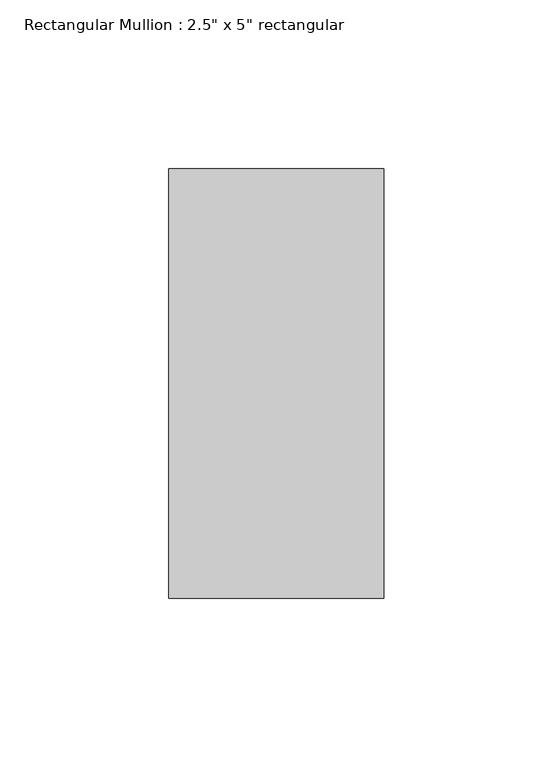
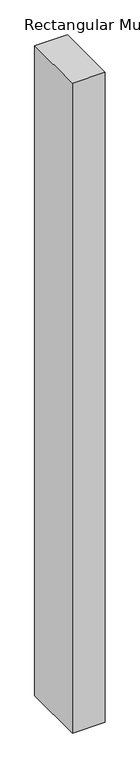
"""IFC4 building model written with IfcOpenShell, lengths in millimetres: member geometry."""

from ifc_helpers import new_model, si_unit, frame, origin, place, context, project, spatial, polyline, outline, extrude, source, transform, mapped, element, save


def member_abf390f1(model_context):
    return source(origin(), model_context, "Body", "SweptSolid", [
        extrude(outline(polyline([(0.0, 63.5), (0.0, -63.5), (-63.5, -63.5), (-63.5, 63.5), (0.0, 63.5)])), frame((0.0, 0.0, -1333.4999998), z_axis=(0.0, 0.0, 1.0), x_axis=(1.0, 0.0, 0.0)), (0.0, 0.0, 1.0), 1333.4999998),
    ])


if __name__ == "__main__":
    model = new_model("IFC4")
    model_context = context("Model", 3, world=origin())
    ifc_project = project(units=[si_unit("LENGTHUNIT", "METRE", prefix="MILLI")], contexts=[model_context])
    site = spatial("IfcSite", under=ifc_project)
    building = spatial("IfcBuilding", under=site)
    placement = place(None, origin())
    member_shape = member_abf390f1(model_context)
    element("IfcMember", 1, ObjectType="Rectangular Mullion : 2.5\" x 5\" rectangular", at=placement, inside=building, context=model_context, shape_type="MappedRepresentation", body=[
        mapped(member_shape, transform((0.0, 0.0, 0.0), x_axis=(1.0, 0.0, 0.0), y_axis=(0.0, 1.0, 0.0), z_axis=(0.0, 0.0, 1.0))),
    ])
    save(model, "model.ifc")

# Revit data of these elements
# Type "Rectangular Mullion : 2.5\" x 5\" rectangular"
#   built-in parameter 1007304 = 0.416667 (stored number, unit not read)
#   built-in parameter 1007301 = 0.104167 (stored number, unit not read)
#   built-in parameter 1007300 = 0.104167 (stored number, unit not read)
# Element 1 (IfcMember, "Rectangular Mullion : 2.5\" x 5\" rectangular")
#   Materials on its faces: "Aluminum"
# Materials
#   "Aluminum": class "Metal", colour RGB 247 247 247, transparency 0, Description = "Aluminum 6061", Cost = 0
